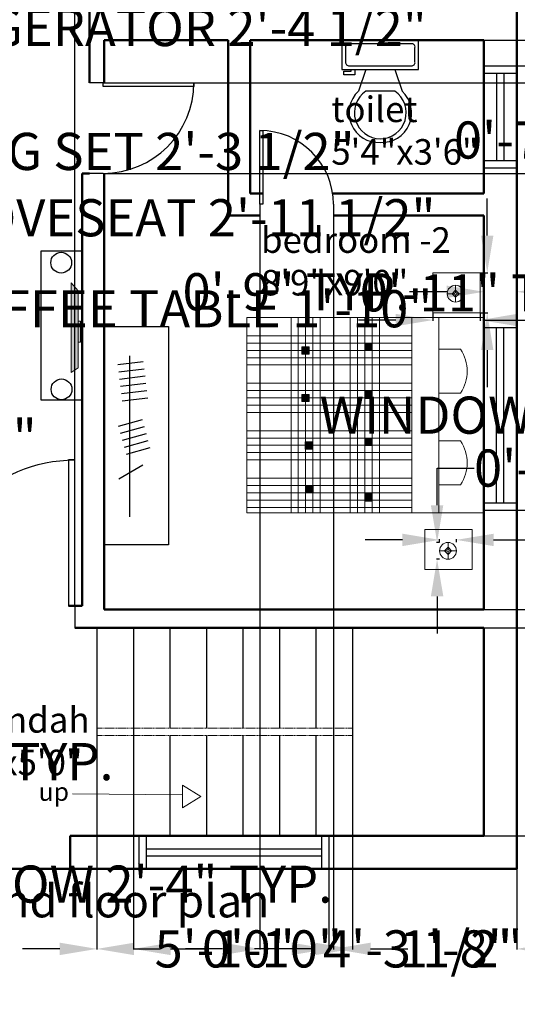
# Model space of a CAD drawing. Units: inches. Extents: x 19 to 1371, y 7 to 588.
# Tile 2 of 5: x 1070 to 1207, y 103 to 372. Entities that reach past the tile are written whole.
import ezdxf

# ---------------------------------------------------------------- set-up
doc = ezdxf.new("R2010")
doc.units = ezdxf.units.IN
doc.header["$MEASUREMENT"] = 0
doc.linetypes.add('DASHED2', pattern=[0.375, 0.25, -0.125])
for name, color, linetype, lineweight in [('A-ANNO-DIMS', 2, 'Continuous', 18), ('A-ANNO-SYMB', 7, 'Continuous', 18), ('A-ANNO-TEXT', 7, 'Continuous', 18), ('A-AREA-IDEN', 7, 'Continuous', 18), ('A-DOOR', 3, 'Continuous', 25), ('A-EQPM', 8, 'Continuous', 18), ('A-FLOR-CABN', 8, 'Continuous', 25), ('A-FLOR-FIXT', 9, 'Continuous', 25), ('A-FLOR-STRS', 7, 'Continuous', 25), ('A-FLOR-STRS-HIDN', 8, 'DASHED2', 18), ('A-FURN', 8, 'Continuous', 18), ('A-FURN-PATT', 252, 'Continuous', 13), ('A-GLAZ', 4, 'Continuous', 25), ('A-WALL', 7, 'Continuous', 50)]:
    doc.layers.add(name, color=color, linetype=linetype, lineweight=lineweight)
doc.styles.get("Standard").update_dxf_attribs({"font": 'arial.ttf'})
doc.dimstyles.get("Standard").update_dxf_attribs({"dimtxt": 10.18, "dimasz": 10.18, "dimexe": 0.18, "dimexo": 0.0625, "dimgap": 0.09, "dimtad": 0, "dimtih": 1, "dimtoh": 1, "dimdec": 0, "dimzin": 0, "dimdsep": 46, "dimlunit": 3, "dimtxsty": 'Standard', "dimcen": 0.09, "dimadec": 0, "dimazin": 0, "dimtfac": 1, "dimtdec": 0, "dimtofl": 0, "dimtmove": 0, "dimatfit": 3, "dimfxl": 1, "dimtolj": 1, "dimtzin": 0, "dimarcsym": 0})

# ---------------------------------------------------------------- blocks, each defined once
blk = doc.blocks.new('*U2')
for p, q in [((0, 0), (0, -6)), ((40, 0), (40, -6))]:
    blk.add_line(p, q)
blk.add_lwpolyline([(0, 0), (0, 40), (1.75, 40), (1.75, 0)], close=True)
blk.add_arc((0, 0), 40, 0, 90)
blk = doc.blocks.new('*U4')
for p, q in [((9.5, -6), (9.5, -2)), ((-8, -8.5), (-8, -8)), ((-7, -8), (-7, -9.5)), ((-4, -8), (-6, -14)), ((4, -8), (6, -14)), ((-10, -8.5), (-8, -8.5)), ((-10, -9.5), (-10, -8.5)), ((-7, -9.5), (-10, -9.5)), ((4, -14), (-4, -14))]:
    blk.add_line(p, q)
blk.add_lwpolyline([(10.5, -8), (10.5, 0), (-10.5, 0), (-10.5, -8)], close=True)
for points in [[(-9.5, -2), (-9.5, -6)], [(8.5, -1), (-8.5, -1)], [(-8.5, -7), (8.5, -7)]]:
    blk.add_lwpolyline(points)
for centre, radius, start, end in [((-8.625, -1.875), 0.8839, 81.8699, 188.1301), ((8.625, -1.875), 0.8839, 351.8699, 98.1301), ((-8.625, -6.125), 0.8839, 171.869898, 278.1301), ((8.625, -6.125), 0.8839, 261.8699, 8.1301), ((-0.4772, -19.9188), 8.0953, 133.01722, 273.38), ((0.0374, -19.8731), 7.127, 124.50543, 269.7), ((-0.0373, -19.8731), 7.127, 270.3, 55.4946), ((0.4773, -19.9188), 8.0953, 266.62, 46.9828)]:
    blk.add_arc(centre, radius, start, end)
blk = doc.blocks.new('Lamp - Table')
for p, q in [((-1, 0), (-7, 0)), ((0, 3), (-3, 0)), ((-3, 0), (0, -3)), ((0, 7), (0, 1)), ((3, 0), (0, 3)), ((0, -3), (3, 0)), ((1, 0), (7, 0)), ((0, -1), (0, -7))]:
    blk.add_line(p, q)
for radius in [7, 1]:
    blk.add_circle((0, 0), radius)
blk = doc.blocks.new('BED-DOUBLE-PLAN')
h = blk.add_hatch(color=256)
h.dxf.hatch_style = 1
h.paths.add_polyline_path([(9, 34.29), (7, 34.29), (7, 32.29), (9, 32.29)])
h = blk.add_hatch(color=256)
h.dxf.hatch_style = 1
h.paths.add_polyline_path([(22.14, 34.29), (20.14, 34.29), (20.14, 32.29), (22.14, 32.29)])
h = blk.add_hatch(color=256)
h.dxf.hatch_style = 1
h.paths.add_polyline_path([(35.09, 34.29), (33.09, 34.29), (33.09, 32.29), (35.09, 32.29)])
h = blk.add_hatch(color=256)
h.dxf.hatch_style = 1
h.paths.add_polyline_path([(50.26, 34.29), (48.26, 34.29), (48.26, 32.29), (50.26, 32.29)])
h = blk.add_hatch(color=256)
h.dxf.hatch_style = 1
h.paths.add_polyline_path([(10.04, 17.06), (8.04, 17.06), (8.04, 15.06), (10.04, 15.06)])
h = blk.add_hatch(color=256)
h.dxf.hatch_style = 1
h.paths.add_polyline_path([(23.04, 17.06), (21.04, 17.06), (21.04, 15.06), (23.04, 15.06)])
h = blk.add_hatch(color=256)
h.dxf.hatch_style = 1
h.paths.add_polyline_path([(36.04, 17.94), (34.04, 17.94), (34.04, 15.94), (36.04, 15.94)])
h = blk.add_hatch(color=256)
h.dxf.hatch_style = 1
h.paths.add_polyline_path([(47.99, 18.12), (45.99, 18.12), (45.99, 16.12), (47.99, 16.12)])
for p, q in [((8.7, 52.54), (8.7, 58.53)), ((20.7, 52.54), (20.7, 58.53)), ((33.82, 52.54), (33.82, 58.53)), ((45.82, 52.54), (45.82, 58.53)), ((53.49, 52.54), (0, 52.54)), ((0, 45.16), (53.49, 45.16)), ((0, 45.16), (5, 45.16)), ((5, 45.16), (5, 0)), ((7, 45.16), (7, 0)), ((9, 45.16), (9, 0)), ((11, 45.16), (11, 0)), ((13, 45.16), (13, 0)), ((18, 45.16), (18, 0)), ((20, 45.16), (20, 0)), ((22, 45.16), (22, 0)), ((24, 45.16), (24, 0)), ((26, 45.16), (26, 0)), ((31, 45.16), (31, 0)), ((33, 45.16), (33, 0)), ((35, 45.16), (35, 0)), ((37, 45.16), (37, 0)), ((39, 45.16), (39, 0)), ((44, 45.16), (44, 0)), ((46, 45.16), (46, 0)), ((48, 45.16), (48, 0)), ((50, 45.16), (50, 0)), ((52, 45.16), (52, 0)), ((0, 36.29), (53.49, 36.29)), ((0, 34.29), (53.49, 34.29)), ((0, 32.29), (53.49, 32.29)), ((0, 30.29), (53.49, 30.29)), ((0, 28.29), (53.49, 28.29)), ((0, 20.08), (53.49, 20.08)), ((0, 18.08), (53.49, 18.08)), ((0, 16.08), (53.49, 16.08)), ((0, 14.08), (53.49, 14.08)), ((0, 12.08), (53.49, 12.08)), ((5, 0), (5, 4.72)), ((5, 4.72), (5, 0))]:
    blk.add_line(p, q)
for points in [[(53.49, 64.91), (0, 64.91), (0, 0), (53.49, 0)], [(7, 34.29), (9, 34.29), (9, 32.29), (7, 32.29)], [(20.14, 34.29), (22.14, 34.29), (22.14, 32.29), (20.14, 32.29)], [(33.09, 34.29), (35.09, 34.29), (35.09, 32.29), (33.09, 32.29)], [(48.26, 34.29), (50.26, 34.29), (50.26, 32.29), (48.26, 32.29)], [(8.04, 17.06), (10.04, 17.06), (10.04, 15.06), (8.04, 15.06)], [(21.04, 17.06), (23.04, 17.06), (23.04, 15.06), (21.04, 15.06)], [(34.04, 17.94), (36.04, 17.94), (36.04, 15.94), (34.04, 15.94)], [(45.99, 18.12), (47.99, 18.12), (47.99, 16.12), (45.99, 16.12)]]:
    blk.add_lwpolyline(points, close=True)
for centre in [(14.7, 49.44), (39.82, 49.44)]:
    blk.add_arc(centre, 10.9, 56.5918, 123.4082)
blk = doc.blocks.new('WIN-24')
for p, q in [((0, 0), (0, 9)), ((2, 0), (2, 9)), ((26, 0), (26, 9)), ((28, 0), (28, 9)), ((2, 5.5), (26, 5.5)), ((2, 3.5), (26, 3.5))]:
    blk.add_line(p, q)
blk = doc.blocks.new('WIN-48')
for p, q in [((0, 9), (0, 0)), ((2, 9), (2, 0)), ((50, 9), (50, 0)), ((52, 9), (52, 0)), ((2, 5.5), (50, 5.5)), ((2, 3.5), (50, 3.5))]:
    blk.add_line(p, q)
blk = doc.blocks.new('TABLE-BEDSIDE')
blk.add_lwpolyline([(0, 11.01), (12.94, 11.01), (12.94, 0), (0, 0)], close=True)
blk = doc.blocks.new('*D22')
at = {"layer": 'A-ANNO-DIMS', "color": 0, "lineweight": -2, "transparency": 16777216}
for p, q in [((1183.48, 292.09), (1183.48, 290.03)), ((1196.42, 292.09), (1196.42, 290.03)), ((1173.3, 290.21), (1163.12, 290.21)), ((1206.6, 290.21), (1216.78, 290.21))]:
    blk.add_line(p, q, dxfattribs=at)
at = {"layer": 'A-ANNO-DIMS', "color": 0, "transparency": 16777216}
for points in [[(1173.3, 291.91), (1173.3, 288.52), (1183.48, 290.21)], [(1206.6, 291.91), (1206.6, 288.52), (1196.42, 290.21)]]:
    blk.add_solid(points, dxfattribs=at)
at = {"layer": 'Defpoints', "color": 0, "transparency": 16777216}
for p in [(1183.48, 292.15), (1196.42, 292.15), (1196.42, 290.21)]:
    blk.add_point(p, dxfattribs=at)
at = {"layer": 'A-ANNO-DIMS', "color": 0, "transparency": 16777216, "insert": (1295.84, 290.21), "char_height": 10.18, "attachment_point": 5}
blk.add_mtext('\\A1;NIGHTSTAND 1\'-1" TYP.', dxfattribs=at)
blk = doc.blocks.new('*D23')
at = {"layer": 'A-ANNO-DIMS', "color": 0, "lineweight": -2, "transparency": 16777216}
for p, q in [((1198.36, 313.34), (1198.36, 323.52)), ((1196.48, 303.16), (1198.54, 303.16)), ((1196.48, 292.15), (1198.54, 292.15)), ((1198.36, 281.97), (1198.36, 271.79))]:
    blk.add_line(p, q, dxfattribs=at)
at = {"layer": 'A-ANNO-DIMS', "color": 0, "transparency": 16777216}
for points in [[(1196.66, 313.34), (1200.05, 313.34), (1198.36, 303.16)], [(1196.66, 281.97), (1200.05, 281.97), (1198.36, 292.15)]]:
    blk.add_solid(points, dxfattribs=at)
at = {"layer": 'Defpoints', "color": 0, "transparency": 16777216}
for p in [(1196.42, 303.16), (1198.36, 303.16), (1196.42, 292.15)]:
    blk.add_point(p, dxfattribs=at)
at = {"layer": 'A-ANNO-DIMS', "color": 0, "transparency": 16777216, "insert": (1198.36, 297.66), "char_height": 10.18, "attachment_point": 5}
blk.add_mtext('\\A1;0\'-11" TYP.', dxfattribs=at)
blk = doc.blocks.new('*D24')
at = {"layer": 'A-ANNO-DIMS', "color": 0, "lineweight": -2, "transparency": 16777216}
for p, q in [((1175.14, 229.99), (1164.96, 229.99)), ((1185.32, 229.36), (1185.32, 230.17)), ((1189.92, 229.36), (1189.92, 230.17)), ((1200.1, 229.99), (1210.28, 229.99))]:
    blk.add_line(p, q, dxfattribs=at)
at = {"layer": 'A-ANNO-DIMS', "color": 0, "transparency": 16777216}
for points in [[(1175.14, 231.68), (1175.14, 228.29), (1185.32, 229.99)], [(1200.1, 231.68), (1200.1, 228.29), (1189.92, 229.99)]]:
    blk.add_solid(points, dxfattribs=at)
at = {"layer": 'Defpoints', "color": 0, "transparency": 16777216}
for p in [(1185.32, 229.3), (1189.92, 229.99), (1189.92, 229.3)]:
    blk.add_point(p, dxfattribs=at)
at = {"layer": 'A-ANNO-DIMS', "color": 0, "transparency": 16777216, "insert": (1274.37, 229.99), "char_height": 10.18, "attachment_point": 5}
blk.add_mtext('\\A1;LAMP 0\'-4 1/2" TYP.', dxfattribs=at)
blk = doc.blocks.new('*D25')
at = {"layer": 'A-ANNO-DIMS', "color": 0, "lineweight": -2, "transparency": 16777216}
for p, q in [((1184.63, 239.48), (1184.63, 249.66)), ((1184.63, 249.66), (1194.81, 249.66)), ((1185.26, 229.3), (1184.45, 229.3)), ((1185.26, 224.7), (1184.45, 224.7)), ((1184.63, 214.52), (1184.63, 204.34))]:
    blk.add_line(p, q, dxfattribs=at)
at = {"layer": 'A-ANNO-DIMS', "color": 0, "transparency": 16777216}
for points in [[(1182.93, 239.48), (1186.33, 239.48), (1184.63, 229.3)], [(1182.93, 214.52), (1186.33, 214.52), (1184.63, 224.7)]]:
    blk.add_solid(points, dxfattribs=at)
at = {"layer": 'Defpoints', "color": 0, "transparency": 16777216}
for p in [(1184.63, 229.3), (1185.32, 229.3), (1185.32, 224.7)]:
    blk.add_point(p, dxfattribs=at)
at = {"layer": 'A-ANNO-DIMS', "color": 0, "transparency": 16777216, "insert": (1237.79, 249.66), "char_height": 10.18, "attachment_point": 5}
blk.add_mtext('\\A1;0\'-4 1/2" TYP.', dxfattribs=at)
blk = doc.blocks.new('*D26')
at = {"layer": 'A-ANNO-DIMS', "color": 0, "lineweight": -2, "transparency": 16777216}
for p, q in [((991.44, 139.83), (991.44, 135.51)), ((1019.44, 139.83), (1019.44, 135.51)), ((1001.62, 135.69), (1009.26, 135.69)), ((1019.44, 135.69), (1029.62, 135.69))]:
    blk.add_line(p, q, dxfattribs=at)
at = {"layer": 'A-ANNO-DIMS', "color": 0, "transparency": 16777216}
for points in [[(1001.62, 137.39), (1001.62, 133.99), (991.44, 135.69)], [(1009.26, 137.39), (1009.26, 133.99), (1019.44, 135.69)]]:
    blk.add_solid(points, dxfattribs=at)
at = {"layer": 'Defpoints', "color": 0, "transparency": 16777216}
for p in [(991.44, 139.89), (1019.44, 139.89), (1019.44, 135.69)]:
    blk.add_point(p, dxfattribs=at)
at = {"layer": 'A-ANNO-DIMS', "color": 0, "transparency": 16777216, "insert": (1094.12, 135.69), "char_height": 10.18, "attachment_point": 5}
blk.add_mtext('\\A1;WINDOW 2\'-4" TYP.', dxfattribs=at)
blk = doc.blocks.new('*D27')
at = {"layer": 'A-ANNO-DIMS', "color": 0, "lineweight": -2, "transparency": 16777216}
for p, q in [((1023.64, 159.07), (1023.64, 169.25)), ((1023.64, 169.25), (1033.82, 169.25)), ((1019.5, 148.89), (1023.82, 148.89)), ((1019.5, 139.89), (1023.82, 139.89)), ((1023.64, 129.71), (1023.64, 119.53))]:
    blk.add_line(p, q, dxfattribs=at)
at = {"layer": 'A-ANNO-DIMS', "color": 0, "transparency": 16777216}
for points in [[(1021.95, 159.07), (1025.34, 159.07), (1023.64, 148.89)], [(1021.95, 129.71), (1025.34, 129.71), (1023.64, 139.89)]]:
    blk.add_solid(points, dxfattribs=at)
at = {"layer": 'Defpoints', "color": 0, "transparency": 16777216}
for p in [(1019.44, 148.89), (1023.64, 148.89), (1019.44, 139.89)]:
    blk.add_point(p, dxfattribs=at)
at = {"layer": 'A-ANNO-DIMS', "color": 0, "transparency": 16777216, "insert": (1064.94, 169.25), "char_height": 10.18, "attachment_point": 5}
blk.add_mtext('\\A1;0\'-9" TYP.', dxfattribs=at)
blk = doc.blocks.new('*D28')
at = {"layer": 'A-ANNO-DIMS', "color": 0, "lineweight": -2, "transparency": 16777216}
for p, q in [((1206.5, 290.16), (1214.42, 290.16)), ((1214.24, 279.98), (1214.24, 269.51)), ((1214.24, 248.34), (1214.24, 258.8)), ((1206.5, 238.16), (1214.42, 238.16))]:
    blk.add_line(p, q, dxfattribs=at)
at = {"layer": 'A-ANNO-DIMS', "color": 0, "transparency": 16777216}
for points in [[(1212.55, 279.98), (1215.94, 279.98), (1214.24, 290.16)], [(1212.55, 248.34), (1215.94, 248.34), (1214.24, 238.16)]]:
    blk.add_solid(points, dxfattribs=at)
at = {"layer": 'Defpoints', "color": 0, "transparency": 16777216}
for p in [(1206.44, 290.16), (1214.24, 290.16), (1206.44, 238.16)]:
    blk.add_point(p, dxfattribs=at)
at = {"layer": 'A-ANNO-DIMS', "color": 0, "transparency": 16777216, "insert": (1214.24, 264.16), "char_height": 10.18, "attachment_point": 5}
blk.add_mtext('\\A1;WINDOW 4\'-4" TYP.', dxfattribs=at)
blk = doc.blocks.new('*D29')
at = {"layer": 'A-ANNO-DIMS', "color": 0, "lineweight": -2, "transparency": 16777216}
for p, q in [((1187.26, 297.96), (1177.08, 297.96)), ((1197.44, 290.22), (1197.44, 298.14)), ((1206.44, 290.22), (1206.44, 298.14)), ((1216.62, 297.96), (1226.8, 297.96))]:
    blk.add_line(p, q, dxfattribs=at)
at = {"layer": 'A-ANNO-DIMS', "color": 0, "transparency": 16777216}
for points in [[(1187.26, 299.65), (1187.26, 296.26), (1197.44, 297.96)], [(1216.62, 299.65), (1216.62, 296.26), (1206.44, 297.96)]]:
    blk.add_solid(points, dxfattribs=at)
at = {"layer": 'Defpoints', "color": 0, "transparency": 16777216}
for p in [(1197.44, 297.96), (1197.44, 290.16), (1206.44, 290.16)]:
    blk.add_point(p, dxfattribs=at)
at = {"layer": 'A-ANNO-DIMS', "color": 0, "transparency": 16777216, "insert": (1145.97, 297.96), "char_height": 10.18, "attachment_point": 5}
blk.add_mtext('\\A1;0\'-9" TYP.', dxfattribs=at)
blk = doc.blocks.new('*D36')
at = {"layer": 'A-ANNO-DIMS', "color": 0, "lineweight": -2, "transparency": 16777216}
for p, q in [((980.44, 374.59), (980.44, 370.17)), ((1009.08, 374.59), (1009.08, 370.17)), ((990.62, 370.35), (998.9, 370.35)), ((1009.08, 370.35), (1019.26, 370.35))]:
    blk.add_line(p, q, dxfattribs=at)
at = {"layer": 'A-ANNO-DIMS', "color": 0, "transparency": 16777216}
for points in [[(990.62, 372.05), (990.62, 368.66), (980.44, 370.35)], [(998.9, 372.05), (998.9, 368.66), (1009.08, 370.35)]]:
    blk.add_solid(points, dxfattribs=at)
at = {"layer": 'Defpoints', "color": 0, "transparency": 16777216}
for p in [(980.44, 374.65), (1009.08, 374.65), (1009.08, 370.35)]:
    blk.add_point(p, dxfattribs=at)
at = {"layer": 'A-ANNO-DIMS', "color": 0, "transparency": 16777216, "insert": (1102.94, 370.35), "char_height": 10.18, "attachment_point": 5}
blk.add_mtext('\\A1;REFRIGERATOR 2\'-4 1/2"', dxfattribs=at)
blk = doc.blocks.new('*D38')
at = {"layer": 'A-ANNO-DIMS', "color": 0, "lineweight": -2, "transparency": 16777216}
for p, q in [((990.01, 340.47), (990.01, 336.23)), ((1017.49, 340.47), (1017.49, 336.23)), ((1000.19, 336.41), (1007.31, 336.41)), ((1017.49, 336.41), (1027.67, 336.41))]:
    blk.add_line(p, q, dxfattribs=at)
at = {"layer": 'A-ANNO-DIMS', "color": 0, "transparency": 16777216}
for points in [[(1000.19, 338.11), (1000.19, 334.72), (990.01, 336.41)], [(1007.31, 338.11), (1007.31, 334.72), (1017.49, 336.41)]]:
    blk.add_solid(points, dxfattribs=at)
at = {"layer": 'Defpoints', "color": 0, "transparency": 16777216}
for p in [(990.01, 340.54), (1017.49, 340.54), (1017.49, 336.41)]:
    blk.add_point(p, dxfattribs=at)
at = {"layer": 'A-ANNO-DIMS', "color": 0, "transparency": 16777216, "insert": (1095.56, 336.41), "char_height": 10.18, "attachment_point": 5}
blk.add_mtext('\\A1;DINING SET 2\'-3 1/2"', dxfattribs=at)
blk = doc.blocks.new('*D42')
at = {"layer": 'A-ANNO-DIMS', "color": 0, "lineweight": -2, "transparency": 16777216}
for p, q in [((1003.24, 312.95), (1003.24, 318.42)), ((1038.94, 312.95), (1038.94, 318.42)), ((1013.42, 318.24), (1028.76, 318.24)), ((1038.94, 318.24), (1049.12, 318.24))]:
    blk.add_line(p, q, dxfattribs=at)
at = {"layer": 'A-ANNO-DIMS', "color": 0, "transparency": 16777216}
for points in [[(1013.42, 319.94), (1013.42, 316.55), (1003.24, 318.24)], [(1028.76, 319.94), (1028.76, 316.55), (1038.94, 318.24)]]:
    blk.add_solid(points, dxfattribs=at)
at = {"layer": 'Defpoints', "color": 0, "transparency": 16777216}
for p in [(1038.94, 318.24), (1003.24, 312.89), (1038.94, 312.89)]:
    blk.add_point(p, dxfattribs=at)
at = {"layer": 'A-ANNO-DIMS', "color": 0, "transparency": 16777216, "insert": (1117.85, 318.24), "char_height": 10.18, "attachment_point": 5}
blk.add_mtext('\\A1;LOVESEAT 2\'-11 1/2"', dxfattribs=at)
blk = doc.blocks.new('*D44')
at = {"layer": 'A-ANNO-DIMS', "color": 0, "lineweight": -2, "transparency": 16777216}
for p, q in [((1031.78, 283.13), (1031.78, 293.31)), ((1031.78, 293.31), (1041.96, 293.31)), ((1028.56, 283.13), (1031.96, 283.13)), ((1031.78, 271.4), (1031.78, 272.95)), ((1028.56, 261.22), (1031.96, 261.22))]:
    blk.add_line(p, q, dxfattribs=at)
at = {"layer": 'A-ANNO-DIMS', "color": 0, "transparency": 16777216}
for points in [[(1030.09, 272.95), (1033.48, 272.95), (1031.78, 283.13)], [(1030.09, 271.4), (1033.48, 271.4), (1031.78, 261.22)]]:
    blk.add_solid(points, dxfattribs=at)
at = {"layer": 'Defpoints', "color": 0, "transparency": 16777216}
for p in [(1028.5, 283.13), (1031.78, 283.13), (1028.5, 261.22)]:
    blk.add_point(p, dxfattribs=at)
at = {"layer": 'A-ANNO-DIMS', "color": 0, "transparency": 16777216, "insert": (1114.8, 293.31), "char_height": 10.18, "attachment_point": 5}
blk.add_mtext('\\A1;COFFEE TABLE 1\'-10"', dxfattribs=at)
blk = doc.blocks.new('*D45')
at = {"layer": 'A-ANNO-DIMS', "color": 0, "lineweight": -2, "transparency": 16777216}
for p, q in [((1006.59, 261.16), (1006.59, 257.76)), ((1028.5, 261.16), (1028.5, 257.76)), ((1016.77, 257.94), (1018.32, 257.94)), ((1028.5, 257.94), (1038.68, 257.94))]:
    blk.add_line(p, q, dxfattribs=at)
at = {"layer": 'A-ANNO-DIMS', "color": 0, "transparency": 16777216}
for points in [[(1016.77, 259.63), (1016.77, 256.24), (1006.59, 257.94)], [(1018.32, 259.63), (1018.32, 256.24), (1028.5, 257.94)]]:
    blk.add_solid(points, dxfattribs=at)
at = {"layer": 'Defpoints', "color": 0, "transparency": 16777216}
for p in [(1006.59, 261.22), (1028.5, 261.22), (1028.5, 257.94)]:
    blk.add_point(p, dxfattribs=at)
at = {"layer": 'A-ANNO-DIMS', "color": 0, "transparency": 16777216, "insert": (1055.77, 257.94), "char_height": 10.18, "attachment_point": 5}
blk.add_mtext('\\A1;1\'-10"', dxfattribs=at)
blk = doc.blocks.new('*D46')
at = {"layer": 'A-ANNO-DIMS', "color": 0, "lineweight": -2, "transparency": 16777216}
for p, q in [((1035.21, 572.84), (1025.03, 572.84)), ((1045.39, 211.95), (1045.39, 573.02)), ((1085.39, 211.95), (1085.39, 573.02)), ((1095.57, 572.84), (1105.75, 572.84))]:
    blk.add_line(p, q, dxfattribs=at)
at = {"layer": 'A-ANNO-DIMS', "color": 0, "transparency": 16777216}
for points in [[(1035.21, 574.54), (1035.21, 571.14), (1045.39, 572.84)], [(1095.57, 574.54), (1095.57, 571.14), (1085.39, 572.84)]]:
    blk.add_solid(points, dxfattribs=at)
at = {"layer": 'Defpoints', "color": 0, "transparency": 16777216}
for p in [(1085.39, 572.84), (1045.39, 211.89), (1085.39, 211.89)]:
    blk.add_point(p, dxfattribs=at)
at = {"layer": 'A-ANNO-DIMS', "color": 0, "transparency": 16777216, "insert": (1065.39, 572.84), "char_height": 10.18, "attachment_point": 5}
blk.add_mtext('\\A1;3\'-4"', dxfattribs=at)
blk = doc.blocks.new('*D47')
at = {"layer": 'A-ANNO-DIMS', "color": 0, "lineweight": -2, "transparency": 16777216}
for p, q in [((987.23, 211.95), (987.23, 573.02)), ((997.41, 572.84), (1019.34, 572.84)), ((1029.52, 211.95), (1029.52, 573.02)), ((1029.52, 572.84), (1039.7, 572.84))]:
    blk.add_line(p, q, dxfattribs=at)
at = {"layer": 'A-ANNO-DIMS', "color": 0, "transparency": 16777216}
for points in [[(997.41, 574.54), (997.41, 571.14), (987.23, 572.84)], [(1019.34, 574.54), (1019.34, 571.14), (1029.52, 572.84)]]:
    blk.add_solid(points, dxfattribs=at)
at = {"layer": 'Defpoints', "color": 0, "transparency": 16777216}
for p in [(1029.52, 572.84), (987.23, 211.89), (1029.52, 211.89)]:
    blk.add_point(p, dxfattribs=at)
at = {"layer": 'A-ANNO-DIMS', "color": 0, "transparency": 16777216, "insert": (1065.17, 572.84), "char_height": 10.18, "attachment_point": 5}
blk.add_mtext('\\A1;3\'-6 1/2"', dxfattribs=at)
blk = doc.blocks.new('*D49')
at = {"layer": 'A-ANNO-DIMS', "color": 0, "lineweight": -2, "transparency": 16777216}
for p, q in [((1228.39, 355.24), (1228.39, 365.42)), ((1228.39, 365.42), (1238.57, 365.42)), ((1093.5, 355.24), (1228.57, 355.24)), ((1228.39, 340.57), (1228.39, 345.06)), ((1093.5, 330.39), (1228.57, 330.39))]:
    blk.add_line(p, q, dxfattribs=at)
at = {"layer": 'A-ANNO-DIMS', "color": 0, "transparency": 16777216}
for points in [[(1226.7, 345.06), (1230.09, 345.06), (1228.39, 355.24)], [(1226.7, 340.57), (1230.09, 340.57), (1228.39, 330.39)]]:
    blk.add_solid(points, dxfattribs=at)
at = {"layer": 'Defpoints', "color": 0, "transparency": 16777216}
for p in [(1093.44, 355.24), (1228.39, 355.24), (1093.44, 330.39)]:
    blk.add_point(p, dxfattribs=at)
at = {"layer": 'A-ANNO-DIMS', "color": 0, "transparency": 16777216, "insert": (1252.28, 365.42), "char_height": 10.18, "attachment_point": 5}
blk.add_mtext('\\A1;2\'-1"', dxfattribs=at)
blk = doc.blocks.new('*D51')
at = {"layer": 'A-ANNO-DIMS', "color": 0, "lineweight": -2, "transparency": 16777216}
for p, q in [((1136.03, 318.83), (1136.03, 117.76)), ((1156.25, 318.83), (1156.25, 117.76)), ((1125.85, 117.94), (1115.67, 117.94)), ((1166.43, 117.94), (1176.61, 117.94))]:
    blk.add_line(p, q, dxfattribs=at)
at = {"layer": 'A-ANNO-DIMS', "color": 0, "transparency": 16777216}
for points in [[(1125.85, 119.64), (1125.85, 116.24), (1136.03, 117.94)], [(1166.43, 119.64), (1166.43, 116.24), (1156.25, 117.94)]]:
    blk.add_solid(points, dxfattribs=at)
at = {"layer": 'Defpoints', "color": 0, "transparency": 16777216}
for p in [(1136.03, 318.89), (1156.25, 318.89), (1156.25, 117.94)]:
    blk.add_point(p, dxfattribs=at)
at = {"layer": 'A-ANNO-DIMS', "color": 0, "transparency": 16777216, "insert": (1189.75, 117.94), "char_height": 10.18, "attachment_point": 5}
blk.add_mtext('\\A1;1\'-8"', dxfattribs=at)
blk = doc.blocks.new('*D52')
at = {"layer": 'A-ANNO-DIMS', "color": 0, "lineweight": -2, "transparency": 16777216}
for p, q in [((1091.44, 148.83), (1091.44, 117.76)), ((1161.44, 148.83), (1161.44, 117.76)), ((1101.62, 117.94), (1108.87, 117.94)), ((1151.26, 117.94), (1144.02, 117.94))]:
    blk.add_line(p, q, dxfattribs=at)
at = {"layer": 'A-ANNO-DIMS', "color": 0, "transparency": 16777216}
for points in [[(1101.62, 119.64), (1101.62, 116.24), (1091.44, 117.94)], [(1151.26, 119.64), (1151.26, 116.24), (1161.44, 117.94)]]:
    blk.add_solid(points, dxfattribs=at)
at = {"layer": 'Defpoints', "color": 0, "transparency": 16777216}
for p in [(1091.44, 148.89), (1161.44, 148.89), (1161.44, 117.94)]:
    blk.add_point(p, dxfattribs=at)
at = {"layer": 'A-ANNO-DIMS', "color": 0, "transparency": 16777216, "insert": (1126.44, 117.94), "char_height": 10.18, "attachment_point": 5}
blk.add_mtext('\\A1;5\'-10"', dxfattribs=at)
blk = doc.blocks.new('*D53')
at = {"layer": 'A-ANNO-DIMS', "color": 0, "lineweight": -2, "transparency": 16777216}
for p, q in [((1091.44, 205.83), (1091.44, 117.76)), ((1101.44, 205.83), (1101.44, 117.76)), ((1081.26, 117.94), (1071.08, 117.94)), ((1111.62, 117.94), (1121.8, 117.94))]:
    blk.add_line(p, q, dxfattribs=at)
at = {"layer": 'A-ANNO-DIMS', "color": 0, "transparency": 16777216}
for points in [[(1081.26, 119.64), (1081.26, 116.24), (1091.44, 117.94)], [(1111.62, 119.64), (1111.62, 116.24), (1101.44, 117.94)]]:
    blk.add_solid(points, dxfattribs=at)
at = {"layer": 'Defpoints', "color": 0, "transparency": 16777216}
for p in [(1091.44, 205.89), (1101.44, 205.89), (1101.44, 117.94)]:
    blk.add_point(p, dxfattribs=at)
at = {"layer": 'A-ANNO-DIMS', "color": 0, "transparency": 16777216, "insert": (1139.38, 117.94), "char_height": 10.18, "attachment_point": 5}
blk.add_mtext('\\A1;0\'-10"', dxfattribs=at)
blk = doc.blocks.new('*D54')
at = {"layer": 'A-ANNO-DIMS', "color": 0, "lineweight": -2, "transparency": 16777216}
for p, q in [((1197.5, 205.89), (1228.57, 205.89)), ((1228.39, 195.71), (1228.39, 182.68)), ((1228.39, 159.07), (1228.39, 172.1)), ((1197.5, 148.89), (1228.57, 148.89))]:
    blk.add_line(p, q, dxfattribs=at)
at = {"layer": 'A-ANNO-DIMS', "color": 0, "transparency": 16777216}
for points in [[(1226.7, 195.71), (1230.09, 195.71), (1228.39, 205.89)], [(1226.7, 159.07), (1230.09, 159.07), (1228.39, 148.89)]]:
    blk.add_solid(points, dxfattribs=at)
at = {"layer": 'Defpoints', "color": 0, "transparency": 16777216}
for p in [(1197.44, 205.89), (1228.39, 205.89), (1197.44, 148.89)]:
    blk.add_point(p, dxfattribs=at)
at = {"layer": 'A-ANNO-DIMS', "color": 0, "transparency": 16777216, "insert": (1228.39, 177.39), "char_height": 10.18, "attachment_point": 5}
blk.add_mtext('\\A1;4\'-9"', dxfattribs=at)
blk = doc.blocks.new('*D62')
at = {"layer": 'A-ANNO-DIMS', "color": 0, "lineweight": -2, "transparency": 16777216}
for p, q in [((1228.39, 377.07), (1228.39, 387.25)), ((1197.5, 366.89), (1228.57, 366.89)), ((1197.5, 359.89), (1228.57, 359.89)), ((1228.39, 349.71), (1228.39, 339.53)), ((1228.39, 339.53), (1218.21, 339.53))]:
    blk.add_line(p, q, dxfattribs=at)
at = {"layer": 'A-ANNO-DIMS', "color": 0, "transparency": 16777216}
for points in [[(1226.7, 377.07), (1230.09, 377.07), (1228.39, 366.89)], [(1226.7, 349.71), (1230.09, 349.71), (1228.39, 359.89)]]:
    blk.add_solid(points, dxfattribs=at)
at = {"layer": 'Defpoints', "color": 0, "transparency": 16777216}
for p in [(1197.44, 366.89), (1197.44, 359.89), (1228.39, 359.89)]:
    blk.add_point(p, dxfattribs=at)
at = {"layer": 'A-ANNO-DIMS', "color": 0, "transparency": 16777216, "insert": (1204.59, 339.53), "char_height": 10.18, "attachment_point": 5}
blk.add_mtext('\\A1;0\'-7"', dxfattribs=at)
blk = doc.blocks.new('*D63')
at = {"layer": 'A-ANNO-DIMS', "color": 0, "lineweight": -2, "transparency": 16777216}
for p, q in [((1228.39, 238.16), (1228.39, 248.34)), ((1228.39, 248.34), (1238.57, 248.34)), ((1197.5, 238.16), (1228.57, 238.16)), ((1228.39, 221.07), (1228.39, 227.98)), ((1197.5, 210.89), (1228.57, 210.89))]:
    blk.add_line(p, q, dxfattribs=at)
at = {"layer": 'A-ANNO-DIMS', "color": 0, "transparency": 16777216}
for points in [[(1226.7, 227.98), (1230.09, 227.98), (1228.39, 238.16)], [(1226.7, 221.07), (1230.09, 221.07), (1228.39, 210.89)]]:
    blk.add_solid(points, dxfattribs=at)
at = {"layer": 'Defpoints', "color": 0, "transparency": 16777216}
for p in [(1197.44, 238.16), (1228.39, 238.16), (1197.44, 210.89)]:
    blk.add_point(p, dxfattribs=at)
at = {"layer": 'A-ANNO-DIMS', "color": 0, "transparency": 16777216, "insert": (1264.14, 248.34), "char_height": 10.18, "attachment_point": 5}
blk.add_mtext('\\A1;2\'-3 1/2"', dxfattribs=at)
blk = doc.blocks.new('*D67')
at = {"layer": 'A-ANNO-DIMS', "color": 0, "lineweight": -2, "transparency": 16777216}
for p, q in [((1154.94, 139.83), (1154.94, 117.76)), ((1206.44, 139.83), (1206.44, 117.76)), ((1144.76, 117.94), (1134.58, 117.94)), ((1216.62, 117.94), (1226.8, 117.94))]:
    blk.add_line(p, q, dxfattribs=at)
at = {"layer": 'A-ANNO-DIMS', "color": 0, "transparency": 16777216}
for points in [[(1144.76, 119.64), (1144.76, 116.24), (1154.94, 117.94)], [(1216.62, 119.64), (1216.62, 116.24), (1206.44, 117.94)]]:
    blk.add_solid(points, dxfattribs=at)
at = {"layer": 'Defpoints', "color": 0, "transparency": 16777216}
for p in [(1154.94, 139.89), (1206.44, 139.89), (1206.44, 117.94)]:
    blk.add_point(p, dxfattribs=at)
at = {"layer": 'A-ANNO-DIMS', "color": 0, "transparency": 16777216, "insert": (1180.69, 117.94), "char_height": 10.18, "attachment_point": 5}
blk.add_mtext('\\A1;4\'-3 1/2"', dxfattribs=at)

msp = doc.modelspace()

# ---------------------------------------------------------------- hatches: boundary and pattern name
at = {"layer": 'A-FURN-PATT'}
h = msp.add_hatch(color=256, dxfattribs=at)
h.dxf.hatch_style = 1
h.paths.add_polyline_path([(1086.34, 298.19), (1084.39, 300.43), (1084.39, 275.85), (1086.34, 277.12)])
h.paths.add_polyline_path([(1086.95, 289.89), (1086.34, 289.89), (1086.34, 284.16), (1086.95, 284.16)])

# ---------------------------------------------------------------- linework, layer by layer
at = {"layer": 'A-ANNO-SYMB'}
for p, q in [((1114.89, 160.16), (1114.89, 162.79)), ((1114.89, 162.79), (1114.89, 156.56)), ((1119.89, 159.67), (1114.89, 162.79)), ((1084.8, 160.43), (1114.89, 160.16)), ((1114.89, 156.56), (1119.89, 159.67))]:
    msp.add_line(p, q, dxfattribs=at)
at = {"layer": 'A-EQPM'}
for p, q in [((1084.39, 300.43), (1084.39, 275.85)), ((1086.34, 298.19), (1084.39, 300.43)), ((1086.34, 277.12), (1086.34, 298.19)), ((1084.39, 275.85), (1086.34, 277.12))]:
    msp.add_line(p, q, dxfattribs=at)
msp.add_lwpolyline([(1086.34, 289.89), (1086.95, 289.89), (1086.95, 284.16), (1086.34, 284.16)], close=True, dxfattribs=at)
at = {"layer": 'A-FLOR-CABN'}
for p, q in [((1093.44, 288.46), (1111.07, 288.46)), ((1111.07, 288.46), (1111.07, 228.67)), ((1097.16, 278.01), (1104.16, 278.88)), ((1100.38, 280.45), (1100.38, 236.32)), ((1097.41, 276.03), (1104.4, 276.89)), ((1097.65, 274.04), (1104.65, 274.91)), ((1097.65, 274.04), (1104.65, 274.91)), ((1097.9, 272.06), (1104.89, 272.92)), ((1098.14, 270.07), (1105.14, 270.94)), ((1098.39, 268.09), (1105.38, 268.95)), ((1097.38, 261.15), (1103.91, 262.98)), ((1097.92, 259.22), (1104.45, 261.05)), ((1098.46, 257.3), (1104.99, 259.13)), ((1099, 255.37), (1105.53, 257.2)), ((1099.54, 253.45), (1106.07, 255.28)), ((1097.48, 246.73), (1104.04, 250.53)), ((1111.07, 228.67), (1093.44, 228.67))]:
    msp.add_line(p, q, dxfattribs=at)
msp.add_lwpolyline([(1087.44, 309.04), (1076.06, 309.04), (1076.06, 268.39), (1087.44, 268.39)], close=True, dxfattribs=at)
for centre in [(1081.66, 305.93), (1081.75, 271.23)]:
    msp.add_circle(centre, 2.84, dxfattribs=at)
at = {"layer": 'A-FLOR-STRS'}
for p, q in [((1091.44, 205.89), (1091.44, 148.89)), ((1101.44, 205.89), (1101.44, 178.39)), ((1111.44, 205.89), (1111.44, 178.39)), ((1111.44, 205.89), (1111.44, 178.39)), ((1121.44, 205.89), (1121.44, 178.39)), ((1131.44, 205.89), (1131.44, 178.39)), ((1141.44, 205.89), (1141.44, 178.39)), ((1141.44, 205.89), (1141.44, 178.39)), ((1151.44, 205.89), (1151.44, 178.39)), ((1161.44, 205.89), (1161.44, 148.89)), ((1101.44, 176.39), (1101.44, 148.89)), ((1111.44, 176.39), (1111.44, 148.89)), ((1111.44, 176.39), (1111.44, 148.89)), ((1121.44, 176.39), (1121.44, 148.89)), ((1131.44, 176.39), (1131.44, 148.89)), ((1141.44, 176.39), (1141.44, 148.89)), ((1141.44, 176.39), (1141.44, 148.89)), ((1151.44, 176.39), (1151.44, 148.89))]:
    msp.add_line(p, q, dxfattribs=at)
at = {"layer": 'A-FLOR-STRS-HIDN'}
for p, q in [((1091.44, 178.39), (1161.44, 178.39)), ((1091.44, 176.39), (1161.44, 176.39))]:
    msp.add_line(p, q, dxfattribs=at)
at = {"layer": 'A-WALL'}
for p, q in [((1206.44, 499.89), (1206.44, 139.89)), ((1089.44, 355.24), (1089.44, 380.02)), ((1093.44, 366.89), (1127.44, 366.89)), ((1093.44, 355.24), (1093.44, 366.89)), ((1127.44, 366.89), (1127.44, 318.89)), ((1133.44, 366.89), (1133.44, 324.89)), ((1133.44, 366.89), (1197.44, 366.89)), ((1197.44, 366.89), (1197.44, 324.89)), ((1087.44, 324.89), (1087.44, 330.39)), ((1087.44, 330.39), (1087.44, 330.39)), ((1089.44, 330.39), (1087.44, 330.39)), ((1093.44, 210.89), (1093.44, 330.39)), ((1087.44, 211.89), (1087.44, 324.89)), ((1133.44, 324.89), (1136.91, 324.89)), ((1156.03, 324.89), (1197.44, 324.89)), ((1127.44, 318.89), (1136.03, 318.89)), ((1156.25, 318.89), (1197.44, 318.89)), ((1197.44, 318.89), (1197.44, 210.89)), ((1083.64, 211.89), (1087.44, 211.89)), ((1093.44, 210.89), (1197.44, 210.89)), ((1085.39, 205.89), (1197.44, 205.89)), ((1197.44, 205.89), (1197.44, 148.89)), ((1197.44, 148.89), (1084.13, 148.89)), ((1084.13, 148.89), (1084.13, 139.89)), ((1041.44, 139.89), (1084.13, 139.89)), ((1206.44, 139.89), (1084.13, 139.89))]:
    msp.add_line(p, q, dxfattribs=at)

# ---------------------------------------------------------------- block references
at = {"layer": 'A-DOOR', "xscale": 0.6212879094378088, "yscale": 0.6212879094378088, "zscale": 0.6212879094378088, "rotation": 270}
msp.add_blockref('*U2', (1093.17, 355.24), dxfattribs=at)
at = {"layer": 'A-DOOR', "xscale": 0.5055103625222516, "yscale": 0.5055103625222516, "zscale": 0.5055103625222516}
msp.add_blockref('*U2', (1136.03, 321.92), dxfattribs=at)
at = {"layer": 'A-DOOR', "xscale": -1}
msp.add_blockref('*U2', (1085.39, 211.89), dxfattribs=at)
at = {"layer": 'A-FLOR-FIXT'}
msp.add_blockref('*U4', (1169.07, 366.89), dxfattribs=at)
at = {"layer": 'A-FURN'}
for p in [(1183.48, 292.15), (1181.26, 221.87)]:
    msp.add_blockref('TABLE-BEDSIDE', p, dxfattribs=at)
at = {"layer": 'A-FURN', "xscale": 0.3285708312946518, "yscale": 0.3285708312946518, "zscale": 0.3285708312946518}
for p in [(1189.7, 297.44), (1187.62, 227)]:
    msp.add_blockref('Lamp - Table', p, dxfattribs=at)
at = {"layer": 'A-FURN', "rotation": 269.9999999999996}
msp.add_blockref('BED-DOUBLE-PLAN', (1132.53, 290.9), dxfattribs=at)
at = {"layer": 'A-GLAZ'}
for name, p, rotation in [('WIN-24', (1197.44, 359.89), 270.0000000000021), ('WIN-48', (1206.44, 238.16), 90.00000000000097)]:
    msp.add_blockref(name, p, dxfattribs=dict(at, rotation=rotation))
msp.add_blockref('WIN-48', (1102.93, 139.89), dxfattribs=at)

# ---------------------------------------------------------------- texts
at = {"layer": 'A-ANNO-TEXT', "attachment_point": 1}
for s, width, insert, char_height in [('up', 13.7684, (1075.45, 163.5), 5), ('ground floor plan', 147.0306, (1038.93, 135.57), 9)]:
    msp.add_mtext_dynamic_manual_height_columns(s, width=width, gutter_width=1, heights=[0], dxfattribs=dict(at, insert=insert, char_height=char_height))
at = {"layer": 'A-AREA-IDEN', "char_height": 7, "attachment_point": 1}
for s, insert in [('toilet\\P5\'4"x3\'6"', (1155.65, 351.45)), ('bedroom -2\\P8\'9"x9\'0"', (1136.4, 315.62)), ('verandah\\P4\'0"x5\'0"', (1047.18, 184.17))]:
    msp.add_mtext_dynamic_manual_height_columns(s, width=53.7683, gutter_width=1, heights=[0], dxfattribs=dict(at, insert=insert))

# ---------------------------------------------------------------- dimensions: what is measured, and where the dimension line sits
at = {"layer": 'A-ANNO-DIMS'}
for base, p1, p2, picture, middle in [((1029.52, 572.84), (987.23, 211.89), (1029.52, 211.89), '*D47', (1065.17, 572.84)), ((1085.39, 572.84), (1045.39, 211.89), (1085.39, 211.89), '*D46', (1065.39, 572.84)), ((1156.25, 117.94), (1136.03, 318.89), (1156.25, 318.89), '*D51', (1189.75, 117.94)), ((1028.5, 257.94), (1006.59, 261.22), (1028.5, 261.22), '*D45', (1055.77, 257.94)), ((1101.44, 117.94), (1091.44, 205.89), (1101.44, 205.89), '*D53', (1139.38, 117.94)), ((1161.44, 117.94), (1091.44, 148.89), (1161.44, 148.89), '*D52', (1126.44, 117.94)), ((1206.44, 117.94), (1154.94, 139.89), (1206.44, 139.89), '*D67', (1180.69, 117.94))]:
    dim = msp.add_linear_dim(base=base, p1=p1, p2=p2, dimstyle='Standard', override={"dimdec": 1, "dimlfac": 1, "dimrnd": 0, "dimzin": 1, "dimdsep": 46, "dimlunit": 4, "dimfrac": 2}, dxfattribs=at)
    dim.commit()
    dim.dimension.update_dxf_attribs({"geometry": picture, "text_midpoint": middle})
for base, p1, p2, text, picture, middle in [((1009.08, 370.35), (980.44, 374.65), (1009.08, 374.65), 'REFRIGERATOR <>', '*D36', (1102.94, 370.35)), ((1017.49, 336.41), (990.01, 340.54), (1017.49, 340.54), 'DINING SET <>', '*D38', (1095.56, 336.41)), ((1038.94, 318.24), (1003.24, 312.89), (1038.94, 312.89), 'LOVESEAT <>', '*D42', (1117.85, 318.24)), ((1196.42, 290.21), (1183.48, 292.15), (1196.42, 292.15), 'NIGHTSTAND <> TYP.', '*D22', (1295.84, 290.21)), ((1189.92, 229.99), (1185.32, 229.3), (1189.92, 229.3), 'LAMP <> TYP.', '*D24', (1274.37, 229.99)), ((1019.44, 135.69), (991.44, 139.89), (1019.44, 139.89), 'WINDOW <> TYP.', '*D26', (1094.12, 135.69))]:
    dim = msp.add_linear_dim(base=base, p1=p1, p2=p2, text=text, dimstyle='Standard', override={"dimdec": 1, "dimlfac": 1, "dimrnd": 0, "dimzin": 1, "dimdsep": 46, "dimlunit": 4, "dimfrac": 2}, dxfattribs=at)
    dim.commit()
    dim.dimension.update_dxf_attribs({"geometry": picture, "text_midpoint": middle})
for base, p1, p2, picture, middle in [((1228.39, 359.89), (1197.44, 366.89), (1197.44, 359.89), '*D62', (1204.59, 339.53)), ((1228.39246, 355.24399), (1093.44246, 330.39396), (1093.44246, 355.24399), '*D49', (1252.27977, 365.42399)), ((1228.39, 238.16), (1197.44, 210.89), (1197.44, 238.16), '*D63', (1264.14, 248.34)), ((1228.39, 205.89), (1197.44, 148.89), (1197.44, 205.89), '*D54', (1228.39, 177.39))]:
    dim = msp.add_linear_dim(base=base, p1=p1, p2=p2, angle=90, dimstyle='Standard', override={"dimdec": 1, "dimlfac": 1, "dimrnd": 0, "dimzin": 1, "dimdsep": 46, "dimlunit": 4, "dimfrac": 2}, dxfattribs=at)
    dim.commit()
    dim.dimension.update_dxf_attribs({"geometry": picture, "text_midpoint": middle})
for base, p1, p2, angle, text, picture, middle in [((1198.36, 303.16), (1196.42, 292.15), (1196.42, 303.16), 90, '<> TYP.', '*D23', (1198.36, 297.66)), ((1031.78, 283.13), (1028.5, 261.22), (1028.5, 283.13), 90, 'COFFEE TABLE <>', '*D44', (1114.8, 293.31)), ((1197.44, 297.96), (1206.44, 290.16), (1197.44, 290.16), 180, '<> TYP.', '*D29', (1145.97, 297.96)), ((1214.24, 290.16), (1206.44, 238.16), (1206.44, 290.16), 90, 'WINDOW <> TYP.', '*D28', (1214.24, 264.16)), ((1184.63, 229.3), (1185.32, 224.7), (1185.32, 229.3), 90, '<> TYP.', '*D25', (1237.79, 249.66)), ((1023.64, 148.89), (1019.44, 139.89), (1019.44, 148.89), 90, '<> TYP.', '*D27', (1064.94, 169.25))]:
    dim = msp.add_linear_dim(base=base, p1=p1, p2=p2, angle=angle, text=text, dimstyle='Standard', override={"dimdec": 1, "dimlfac": 1, "dimrnd": 0, "dimzin": 1, "dimdsep": 46, "dimlunit": 4, "dimfrac": 2}, dxfattribs=at)
    dim.commit()
    dim.dimension.update_dxf_attribs({"geometry": picture, "text_midpoint": middle})

doc.saveas('drawing.dxf')
